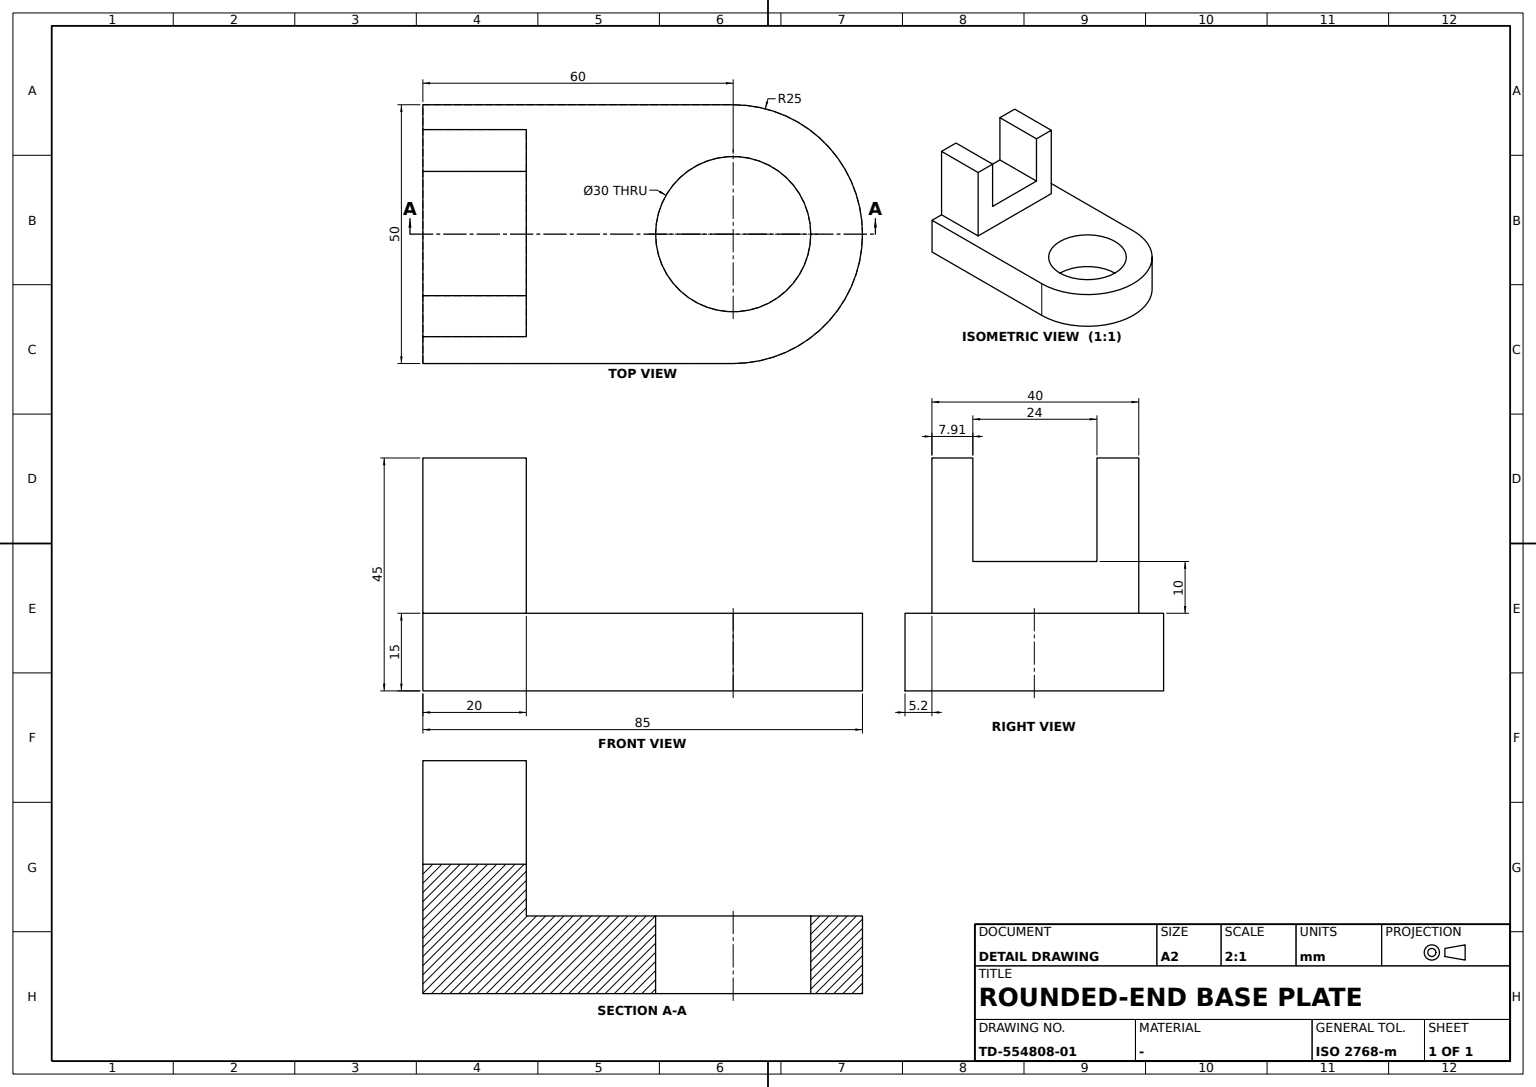
CATIA V5 part; units mm, degrees
sketch "Sketch1" plane through (0, 0, 0) normal (0, 0, 1) x (0, 1, 0)
  arc A0 (-25, 0) -> (25, 0) centre (0, 0) ccw
  point P0 (-25, 0)
  line L0 (-25, 0) -> (-25, 60)
  point P1 (-25, 60)
  point P2 (25, 60)
  point P3 (25, 0)
  line L1 (25, 0) -> (25, 60)
  line L2 (-25, 60) -> (25, 60)
  point P4 (-25, 0)
  point P5 (25, 0)
  dimension "radius A0" = 25
  dimension "length L1" = 60
  constraint coincidence P0 A0
  constraint coincidence P0 x-axis
  constraint coincidence L1 P5
  constraint coincidence L0 P4
  constraint coincidence P0 P4
  constraint coincidence P3 P5
  constraint tangency L0 A0
  constraint symmetry P1 P2 y-axis
  constraint symmetry P0 P3 y-axis
  constraint symmetry L0 L1 y-axis
  constraint horizontal L2 x-axis
extrude "Pad1" add sketch "Sketch1" along normal blind 15
sketch "Sketch2" plane through (-60, 0, 0) normal (-1, 0, 0) x (0, -1, 0)
  line L0 (-20.1983, 15) -> (19.8017, 15)
  line L1 (19.8017, 15) -> (19.8017, 45)
  line L2 (19.8017, 45) -> (11.8872, 45)
  line L3 (11.8872, 45) -> (11.8872, 25)
  line L4 (11.8872, 25) -> (-12.1128, 25)
  line L5 (-12.1128, 25) -> (-12.1128, 45)
  point P0 (-12.1128, 45)
  line L6 (-12.1128, 45) -> (-20.1983, 45)
  line L7 (-20.1983, 45) -> (-20.1983, 15)
  dimension "distance L1 L7" = 40
  dimension "distance L3 L5" = 24
  dimension "length L5" = 20
  constraint horizontal L0 x-axis
  constraint horizontal L2 x-axis
  constraint horizontal L4 x-axis
  constraint horizontal L6 x-axis
  constraint vertical L1 y-axis
  constraint vertical L3 y-axis
  constraint vertical L5 y-axis
  constraint vertical L7 y-axis
  constraint coincidence P0 L2
extrude "Pad2" add sketch "Sketch2" against normal blind 20
sketch "Sketch3" plane through (12.093, -2.3041, 15) normal (0, 0, 1) x (1, 0, 0)
  point P0 (-12.093, 2.3041)
  arc A0 (-12.093, -22.6959) -> (-12.093, 27.3041) centre (-12.093, 2.3041) ccw construction
  constraint concentricity A0 P0
hole "Hole1" at (0, 0, 15) direction (0, 0, -1) diameter 30 end up to next
properties part number "catia 8"
